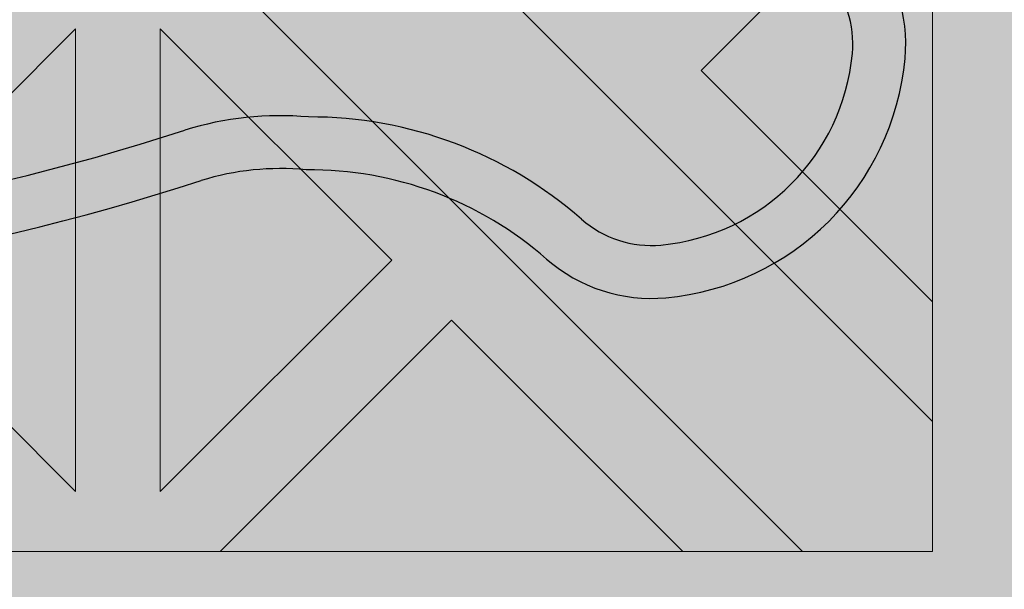
# Model space of a CAD drawing. Units: inches. Extents: x 844 to 2234, y 346 to 1084.
# Tile 10 of 93: x 1124.57 to 1127.536, y 686.542 to 688.258. Entities that reach past the tile are written whole.
import ezdxf

# ---------------------------------------------------------------- set-up
doc = ezdxf.new("R2010")
doc.units = ezdxf.units.IN
doc.header["$MEASUREMENT"] = 0
for name, color, linetype, lineweight in [('A-ANNO-DIMS', 2, 'Continuous', 18), ('furniture', 8, 'Continuous', 18), ('RA-AP-01$0$INT', 35, 'Continuous', 5)]:
    doc.layers.add(name, color=color, linetype=linetype, lineweight=lineweight)
doc.layers.add('RA-AP-01$0$FURN', color=3, linetype='Continuous')
doc.layers.add('RA-AP-01$0$WOOD', color=64, linetype='Continuous')
doc.styles.get("Standard").update_dxf_attribs({"font": 'arial.ttf'})
doc.dimstyles.get("Standard").update_dxf_attribs({"dimtxt": 6, "dimasz": 3, "dimexe": 0.18, "dimexo": 0.0625, "dimgap": 0.09, "dimtad": 0, "dimtih": 1, "dimtoh": 1, "dimdec": 1, "dimzin": 0, "dimdsep": 46, "dimlunit": 3, "dimtxsty": 'Standard', "dimblk": 'ARCHTICK', "dimcen": 0.09, "dimadec": 0, "dimazin": 0, "dimtfac": 1, "dimtdec": 1, "dimtofl": 0, "dimtmove": 0, "dimatfit": 3, "dimfxl": 1, "dimtolj": 1, "dimtzin": 0, "dimarcsym": 0})

# ---------------------------------------------------------------- blocks, each defined once
blk = doc.blocks.new('A$C18D01794')
at = {"layer": 'RA-AP-01$0$INT'}
blk.add_hatch(color=256, dxfattribs=at).paths.add_polyline_path([(4.505206456958071, -6.306712009588038), (5.305206456958072, -6.306712009588038), (5.305206456958072, -7.106712009588038), (5.255206456951893, -7.10671200958804), (5.25520645694868, -6.356712009605972), (4.555206456959269, -6.356712009587461), (4.555206456956052, -7.106712009588038), (4.505206456958073, -7.106712009588038)])
h = blk.add_hatch(color=256, dxfattribs=at)
h.paths.add_polyline_path([(4.585917135068449, -6.356712009588271), (4.555206456959269, -6.35671200958746), (4.555206456959137, -6.387422687716308), (4.874495778835233, -6.706712009592356), (4.90520645695423, -6.676001331474049)])
h.paths.add_polyline_path([(5.255206456948813, -6.387422687716306), (5.255206456948682, -6.356712009605972), (5.224495778822613, -6.356712009605161), (4.905206456953498, -6.676001331474273), (4.935917135072151, -6.706712009592924)])
h.paths.add_polyline_path([(4.935917135072559, -6.706712009592068), (4.905206456953564, -6.737422687710376), (5.255206456951813, -7.087422687708613), (5.255206456951549, -7.026001331471008)])
h.paths.add_polyline_path([(4.555206456956399, -7.026001331471013), (4.555206456956134, -7.087422687708616), (4.905206456953821, -6.737422687710943), (4.874495778835166, -6.70671200959229)])
h = blk.add_hatch(color=256, dxfattribs=at)
h.paths.add_polyline_path([(4.585917135068448, -6.356712009588273), (4.614201406330596, -6.356712009589021), (4.668846067270487, -6.411356670531338), (4.723490728212344, -6.356712009591912), (4.771774999457151, -6.35671200959319), (4.826419660396886, -6.411356670535356), (4.862780050090322, -6.374996280843536), (4.844495778842715, -6.356712009595112), (4.862780050090411, -6.356712009595595), (4.905206456960182, -6.399138416468211), (4.947632863832445, -6.356712009597838), (4.965917135079675, -6.356712009598322), (4.947632863831759, -6.374996280845421), (4.983993253523576, -6.411356670538857), (5.038637914464627, -6.356712009600247), (5.08692218571208, -6.356712009601523), (5.141566846649976, -6.411356670541852), (5.196211507589851, -6.356712009604411), (5.224495778822615, -6.356712009605161), (4.905206456953975, -6.676001331473793)])
h.paths.add_polyline_path([(4.895206456956031, -6.637717060225675), (4.895206456958921, -6.528427738347902), (4.840561796018589, -6.583072399285802)], flags=16)
h.paths.add_polyline_path([(4.915206456955638, -6.637717060226121), (4.969851117895509, -6.583072399288678), (4.915206456957609, -6.528427738348344)], flags=16)
h.paths.add_polyline_path([(4.826419660395175, -6.568930263661755), (4.881064321335613, -6.514285602723745), (4.771774999456703, -6.514285602720857)], flags=16)
h.paths.add_polyline_path([(4.983993253519558, -6.568930263665262), (5.038637914460456, -6.514285602726792), (4.929348592581548, -6.514285602724816)], flags=16)
h.paths.add_polyline_path([(4.881064321336025, -6.494285602723742), (4.826419660397532, -6.439640941782821), (4.771774999457062, -6.494285602720859)], flags=16)
h.paths.add_polyline_path([(4.929348592582019, -6.494285602724817), (5.038637914460982, -6.494285602726792), (4.983993253522945, -6.439640941786327)], flags=16)
h.paths.add_polyline_path([(4.895206456960191, -6.480143467100443), (4.895206456962115, -6.407422687715913), (4.876922185715016, -6.389138416467584), (4.840561796021581, -6.425498806159401)], flags=16)
h.paths.add_polyline_path([(4.915206456958487, -6.480143467100889), (4.969851117899527, -6.425498806162279), (4.933490728206909, -6.389138416468043), (4.9152064569598, -6.40742268771434)], flags=16)
h.paths.add_polyline_path([(4.757632863832376, -6.480143467096812), (4.812277524772842, -6.425498806158772), (4.757632863834348, -6.370854145217844)], flags=16)
h.paths.add_polyline_path([(4.737632863832376, -6.480143467096286), (4.737632863834348, -6.370854145217375), (4.682988202893906, -6.425498806155385)], flags=16)
h.paths.add_polyline_path([(5.05278005008503, -6.480143467103376), (5.052780050087917, -6.370854145224413), (4.998135389146995, -6.425498806162908)], flags=16)
h.paths.add_polyline_path([(5.072780050085024, -6.480143467103744), (5.127424711025931, -6.42549880616527), (5.072780050087916, -6.370854145224832)], flags=16)
h.paths.add_polyline_path([(4.935917135072783, -6.706712009592292), (5.255206456948811, -6.387422687716309), (5.255206456948932, -6.415706958964177), (5.200561796010279, -6.470351619902839), (5.255206456949403, -6.524996280841948), (5.25520645694961, -6.5732805520894), (5.200561796009787, -6.627925213029239), (5.236922185702417, -6.664285602721864), (5.255206456949919, -6.646001331474357), (5.255206456949998, -6.664285602721898), (5.212780050078687, -6.706712009592262), (5.25520645695036, -6.749138416463932), (5.255206456950438, -6.767422687711313), (5.236922185702424, -6.749138416463297), (5.200561796009796, -6.785498806155928), (5.255206456950753, -6.840143467096874), (5.25520645695096, -6.888427738341682), (5.200561796010322, -6.943072399282328), (5.255206456951428, -6.997717060223427), (5.255206456951547, -7.026001331471006)])
h.paths.add_polyline_path([(5.042988202883395, -6.785498806155427), (5.097632863823085, -6.840143467095101), (5.097632863822622, -6.730854145216193)], flags=16)
h.paths.add_polyline_path([(5.028846067259663, -6.771356670531693), (5.083490728198774, -6.716712009592573), (4.974201406321001, -6.716712009593042)], flags=16)
h.paths.add_polyline_path([(5.117632863823087, -6.840143467095186), (5.172277524762331, -6.785498806155926), (5.11763286382262, -6.730854145216225)], flags=16)
h.paths.add_polyline_path([(5.08349072819877, -6.696712009593886), (5.028846067259652, -6.642067348654775), (4.974201406320998, -6.696712009593438)], flags=16)
h.paths.add_polyline_path([(5.131774999446817, -6.854285602718917), (5.186419660386065, -6.799640941779662), (5.241064321325782, -6.854285602719365)], flags=17)
h.paths.add_polyline_path([(5.131774999446228, -6.716712009592374), (5.186419660386065, -6.771356670532194), (5.222780050079488, -6.734996280838764), (5.204495778832781, -6.716712009592063)], flags=16)
h.paths.add_polyline_path([(5.097632863822613, -6.682569873970264), (5.097632863823061, -6.573280552091354), (5.042988202883383, -6.627925213031044)], flags=16)
h.paths.add_polyline_path([(5.131774999446899, -6.874285602718915), (5.241064321325809, -6.874285602719364), (5.186419660386591, -6.928930263658598)], flags=17)
h.paths.add_polyline_path([(5.131774999446226, -6.696712009594078), (5.204495778830767, -6.696712009594374), (5.22278005007868, -6.67842773834687), (5.186419660386049, -6.642067348654249)], flags=16)
h.paths.add_polyline_path([(5.11763286382262, -6.682569873970225), (5.17227752476232, -6.627925213030515), (5.117632863823064, -6.573280552091267)], flags=16)
h.paths.add_polyline_path([(5.186419660386069, -6.613783077405491), (5.241064321325754, -6.559138416465795), (5.131774999446791, -6.559138416466263)], flags=16)
h.paths.add_polyline_path([(5.131774999446872, -6.539138416466263), (5.24106432132578, -6.539138416465794), (5.186419660386554, -6.484493755526573)], flags=16)
h.paths.add_polyline_path([(5.255206456951811, -7.08742268770861), (5.255206456951895, -7.106712009588038), (4.555206456956052, -7.106712009588038), (4.555206456956136, -7.087422687708617), (4.905206456953973, -6.737422687710788)])
h.paths.add_polyline_path([(4.983993253513404, -6.8444937555241), (4.92934859257295, -6.899138416462108), (5.03863791445186, -6.899138416465014)], flags=16)
h.paths.add_polyline_path([(4.969851117889988, -6.83035161990006), (4.915206456952556, -6.775706958960171), (4.915206456949648, -6.884996280837944)], flags=16)
h.paths.add_polyline_path([(4.929348592572535, -6.919138416462105), (4.983993253511019, -6.973783077403037), (5.038637914451496, -6.919138416465012)], flags=16)
h.paths.add_polyline_path([(5.052780050074912, -6.93328055208906), (4.998135389134438, -6.987925213027088), (5.052780050072919, -7.042569873968025)], flags=16)
h.paths.add_polyline_path([(5.07278005007491, -6.933280552089588), (5.072780050072918, -7.042569873968497), (5.127424711013374, -6.987925213030498)], flags=16)
h.paths.add_polyline_path([(4.89520645695295, -6.775706958959721), (4.840561796013067, -6.830351619897157), (4.895206456950961, -6.884996280837494)], flags=16)
h.paths.add_polyline_path([(4.915206456948365, -6.933280552085403), (4.915206456946434, -7.006001331471951), (4.933490728192729, -7.024285602719066), (4.969851117886972, -6.987925213026453)], flags=16)
h.paths.add_polyline_path([(4.881064321327021, -6.899138416461022), (4.82641966038902, -6.84449375552057), (4.771774999448108, -6.899138416459029)], flags=16)
h.paths.add_polyline_path([(4.895206456950073, -6.933280552084951), (4.840561796009022, -6.987925213023558), (4.876922185700835, -7.024285602716997), (4.895206456948749, -7.006001331469487)], flags=16)
h.paths.add_polyline_path([(4.983993253510392, -7.0020673486505), (4.947632863816944, -7.038427738342319), (4.965917135064043, -7.05671200959023), (5.038637914448995, -7.056712009591555)], flags=16)
h.paths.add_polyline_path([(4.881064321326543, -6.91913841646102), (4.771774999447578, -6.919138416459031), (4.826419660385607, -6.973783077399508)], flags=16)
h.paths.add_polyline_path([(4.905206456946447, -7.014285602717636), (4.862780050074785, -7.056712009588352), (4.947632863816685, -7.056712009589775)], flags=16)
h.paths.add_polyline_path([(5.14156684663679, -7.002067348654549), (5.086922185696452, -7.056712009592438), (5.196211507574223, -7.056712009594425)], flags=16)
h.paths.add_polyline_path([(4.8264196603837, -7.002067348646972), (4.771774999442643, -7.056712009585575), (4.8444957788276, -7.056712009587508), (4.862780050075511, -7.038427738340416)], flags=16)
h.paths.add_polyline_path([(4.812277524760289, -6.98792521302292), (4.757632863822258, -6.933280552082447), (4.757632863819352, -7.042569873961408)], flags=16)
h.paths.add_polyline_path([(4.73763286382226, -6.933280552082079), (4.682988202881349, -6.987925213020536), (4.737632863819352, -7.04256987396099)], flags=16)
h.paths.add_polyline_path([(4.723490728195188, -7.056712009584289), (4.668846067257299, -7.002067348643949), (4.614201406317417, -7.056712009581383)], flags=16)
h.paths.add_polyline_path([(4.597632863829262, -6.706712009592262), (4.555206456957951, -6.664285602721896), (4.555206456958029, -6.646001331474357), (4.573490728205535, -6.664285602721864), (4.609851117898167, -6.627925213029238), (4.555206456958338, -6.573280552089402), (4.555206456958546, -6.524996280841952), (4.60985111789767, -6.470351619902839), (4.555206456959015, -6.415706958964177), (4.555206456959138, -6.387422687716309), (4.874495778835167, -6.70671200959229), (4.5552064569564, -7.026001331471015), (4.555206456956523, -6.997717060223433), (4.609851117897629, -6.94307239928233), (4.555206456956988, -6.888427738341681), (4.555206456957198, -6.840143467096881), (4.609851117898153, -6.78549880615593), (4.573490728205528, -6.749138416463297), (4.555206456957507, -6.76742268771132), (4.555206456957585, -6.749138416463933)])
h.paths.add_polyline_path([(4.712780050085332, -6.730854145216195), (4.712780050084863, -6.840143467095105), (4.767424711024555, -6.785498806155427)], flags=16)
h.paths.add_polyline_path([(4.726922185709173, -6.716712009592573), (4.781566846648288, -6.771356670531693), (4.836211507586949, -6.716712009593043)], flags=16)
h.paths.add_polyline_path([(4.692780050085327, -6.730854145216225), (4.638135389145619, -6.785498806155928), (4.692780050084865, -6.840143467095185)], flags=16)
h.paths.add_polyline_path([(4.726922185709182, -6.696712009593886), (4.836211507586949, -6.696712009593436), (4.7815668466483, -6.642067348654773)], flags=16)
h.paths.add_polyline_path([(4.678637914461726, -6.71671200959237), (4.605917135075169, -6.716712009592063), (4.587632863828464, -6.734996280838766), (4.623993253521887, -6.771356670532195)], flags=16)
h.paths.add_polyline_path([(4.712780050085336, -6.68256987397026), (4.767424711024568, -6.627925213031042), (4.71278005008489, -6.573280552091352)], flags=16)
h.paths.add_polyline_path([(4.678637914461726, -6.696712009594076), (4.623993253521899, -6.642067348654247), (4.587632863829271, -6.67842773834687), (4.605917135077185, -6.696712009594376)], flags=16)
h.paths.add_polyline_path([(4.692780050085336, -6.682569873970228), (4.692780050084889, -6.573280552091267), (4.638135389145632, -6.627925213030515)], flags=16)
h.paths.add_polyline_path([(4.623993253521885, -6.799640941779662), (4.678637914461131, -6.854285602718915), (4.56934859258217, -6.854285602719365)], flags=17)
h.paths.add_polyline_path([(4.623993253521901, -6.613783077405509), (4.678637914461158, -6.559138416466263), (4.569348592582195, -6.559138416465795)], flags=16)
h.paths.add_polyline_path([(4.678637914461051, -6.874285602718915), (4.623993253521361, -6.928930263658598), (4.569348592582143, -6.874285602719364)], flags=17)
h.paths.add_polyline_path([(4.678637914461076, -6.539138416466263), (4.623993253521399, -6.484493755526573), (4.569348592582167, -6.539138416465796)], flags=16)
h = blk.add_hatch(color=256, dxfattribs=at)
h.paths.add_polyline_path([(4.969851117891331, -6.583072399286455), (4.915206456952669, -6.63771706022511), (4.915206456952222, -6.528427738347337)])
h.paths.add_polyline_path([(4.895206456953064, -6.637717060225108), (4.840561796014413, -6.583072399286448), (4.895206456953533, -6.528427738347335)])
h.paths.add_polyline_path([(4.826419660390684, -6.568930263662714), (4.771774999451003, -6.514285602723024), (4.881064321329913, -6.514285602723489)])
h.paths.add_polyline_path([(4.881064321329884, -6.494285602723492), (4.771774999450921, -6.494285602723024), (4.82641966039018, -6.439640941783778)])
h.paths.add_polyline_path([(4.895206456953734, -6.48014346709988), (4.840561796013912, -6.425498806160046), (4.876922185707337, -6.389138416466622), (4.895206456954043, -6.40742268771333)])
h.paths.add_polyline_path([(4.862780050082808, -6.374996280843689), (4.826419660390178, -6.411356670536314), (4.771774999450351, -6.356712009596481), (4.844495778835303, -6.356712009596181)])
h.paths.add_polyline_path([(4.812277524766446, -6.425498806160041), (4.757632863827191, -6.480143467099289), (4.757632863826741, -6.370854145220329)])
h.paths.add_polyline_path([(4.737632863827191, -6.480143467099214), (4.682988202887508, -6.425498806159518), (4.737632863826743, -6.370854145220299)])
h.paths.add_polyline_path([(4.668846067263777, -6.41135667053579), (4.614201406325123, -6.356712009597128), (4.723490728202894, -6.356712009596675)])
h.paths.add_polyline_path([(4.905206456953846, -6.399138416467422), (4.862780050082654, -6.356712009596229), (4.947632863824561, -6.356712009595756)])
h.paths.add_polyline_path([(4.915206456952028, -6.480143467099882), (4.91520645695173, -6.407422687715346), (4.933490728199234, -6.389138416467428), (4.96985111789186, -6.425498806160055)])
h.paths.add_polyline_path([(5.038637914454841, -6.494285602723048), (4.929348592575874, -6.494285602723497), (4.983993253515593, -6.439640941783787)])
h.paths.add_polyline_path([(4.983993253515065, -6.568930263662725), (4.929348592575849, -6.514285602723495), (5.038637914454755, -6.514285602723045)])
h.paths.add_polyline_path([(5.052780050079843, -6.480143467099317), (4.998135389140595, -6.425498806160058), (5.052780050080309, -6.370854145220356)])
h.paths.add_polyline_path([(4.983993253516868, -6.411356670536324), (4.947632863824241, -6.374996280843694), (4.965917135071747, -6.356712009596188), (5.038637914456701, -6.356712009596504)])
h.paths.add_polyline_path([(5.127424711019533, -6.425498806159557), (5.072780050079843, -6.480143467099239), (5.07278005008031, -6.370854145220326)])
h.paths.add_polyline_path([(5.141566846643269, -6.411356670535829), (5.086922185704154, -6.356712009596707), (5.196211507581929, -6.356712009597176)])
h = blk.add_hatch(color=256, dxfattribs=at)
h.paths.add_polyline_path([(5.028846067259997, -6.642067348655121), (4.974201406321342, -6.696712009593783), (5.083490728199115, -6.69671200959423)])
h.paths.add_polyline_path([(4.974201406321344, -6.716712009593388), (5.028846067260004, -6.771356670532039), (5.083490728199117, -6.716712009592919)])
h.paths.add_polyline_path([(5.042988202883738, -6.785498806155768), (5.097632863823428, -6.840143467095449), (5.097632863822963, -6.73085414521654)])
h.paths.add_polyline_path([(5.117632863822961, -6.730854145216568), (5.117632863823428, -6.840143467095531), (5.172277524762674, -6.785498806156272)])
h.paths.add_polyline_path([(5.131774999446572, -6.716712009592718), (5.186419660386406, -6.77135667053254), (5.222780050079831, -6.734996280839116), (5.204495778833122, -6.716712009592409)])
h.paths.add_polyline_path([(5.236922185702764, -6.749138416463644), (5.200561796010139, -6.785498806156274), (5.255206456949971, -6.840143467096101), (5.255206456950271, -6.76742268771115)])
h.paths.add_polyline_path([(5.186419660386412, -6.799640941780006), (5.131774999447164, -6.854285602719262), (5.241064321326123, -6.854285602719711)])
h.paths.add_polyline_path([(5.131774999447238, -6.874285602719261), (5.186419660386934, -6.928930263658944), (5.241064321326153, -6.874285602719709)])
h.paths.add_polyline_path([(5.200561796010663, -6.943072399282675), (5.255206456949324, -6.997717060221329), (5.255206456949777, -6.888427738343558)])
h.paths.add_polyline_path([(5.21278005007903, -6.706712009592607), (5.255206456950223, -6.749138416463798), (5.255206456950696, -6.664285602721891)])
h.paths.add_polyline_path([(5.13177499944657, -6.696712009594424), (5.204495778831106, -6.696712009594723), (5.222780050079024, -6.678427738347219), (5.186419660386397, -6.642067348654592)])
h.paths.add_polyline_path([(5.117632863823405, -6.573280552091611), (5.117632863822955, -6.682569873970578), (5.172277524762665, -6.627925213030859)])
h.paths.add_polyline_path([(5.042988202883727, -6.627925213031387), (5.097632863822957, -6.682569873970603), (5.097632863823407, -6.573280552091697)])
h.paths.add_polyline_path([(5.131774999447135, -6.559138416466609), (5.186419660386394, -6.613783077405857), (5.241064321326097, -6.559138416466144)])
h.paths.add_polyline_path([(5.200561796010128, -6.627925213029584), (5.236922185702758, -6.664285602722211), (5.255206456950264, -6.646001331474705), (5.255206456949948, -6.573280552089752)])
h.paths.add_polyline_path([(5.186419660386895, -6.484493755526919), (5.131774999447213, -6.539138416466609), (5.241064321326127, -6.539138416466142)])
h.paths.add_polyline_path([(5.200561796010624, -6.470351619903183), (5.255206456949745, -6.524996280842298), (5.255206456949276, -6.415706958964523)])
for p, q in [((4.555206456959269, -6.356712009587461), (5.255206456948681, -6.356712009605972)), ((4.905206456953975, -6.676001331473793), (5.224495778822613, -6.356712009605161)), ((5.086922185712082, -6.356712009601526), (5.141566846649976, -6.411356670541854)), ((5.196211507589851, -6.356712009604413), (5.141566846649976, -6.411356670541854)), ((5.255206456951895, -7.106712009588038), (5.255206456948681, -6.356712009605972)), ((5.052780050087917, -6.370854145224413), (4.998135389146995, -6.425498806162908)), ((5.052780050085028, -6.480143467103376), (5.052780050087917, -6.370854145224413)), ((5.072780050085028, -6.48014346710374), (5.072780050087916, -6.37085414522483)), ((5.072780050087916, -6.37085414522483), (5.127424711025931, -6.42549880616527)), ((4.935917135072783, -6.706712009592292), (5.255206456948813, -6.387422687716307)), ((5.255206456948934, -6.415706958964177), (5.200561796010281, -6.470351619902839)), ((5.052780050085028, -6.480143467103376), (4.998135389146995, -6.425498806162908)), ((5.12742471102593, -6.425498806165272), (5.072780050085028, -6.48014346710374)), ((5.255206456949399, -6.524996280841946), (5.200561796010281, -6.470351619902839))]:
    blk.add_line(p, q, dxfattribs=at)
blk = doc.blocks.new('A$C32926AE1')
at = {"layer": 'RA-AP-01$0$WOOD'}
h = blk.add_hatch(color=256, dxfattribs=at)
h.dxf.hatch_style = 1
h.paths.add_polyline_path([(5.157430609644524, 4.573483066760929, -0.1009492694046607), (5.155401577623758, 4.593365984175333, -0.1842662638101597), (5.172249623284174, 4.638795604568598, 0.2056608120311276), (5.179560981299304, 4.661316324430096, 0.3614336704623542), (5.134352340494423, 4.706524965234944, 0.2056608120311297), (5.111831620632933, 4.699213607219793, -0.1842662638101113), (5.066402000239693, 4.682365561559342, -0.1055311479399994), (5.045656153913092, 4.68467289944697, 0.1567636581983829), (4.763886414745334, 4.684672899446966, -0.1055311479399895), (4.743140568418733, 4.68236556155934, -0.1842662638100833), (4.6977109480255, 4.69921360721979, 0.2056608120302612), (4.675190228164109, 4.706524965234949, 0.3614336704708441), (4.629981587358889, 4.66131632442871, 0.2056608120245944), (4.637292945374126, 4.638795604567974, -0.1842662638101024), (4.654140991034615, 4.59336598417475, -0.1009492694055169), (4.652111959013835, 4.573483066760181, 0.021410119221476), (4.629748025606143, 4.156712009541676, 0.0214101192214795), (4.652111959013809, 3.739940952323101, -0.1009492694059586), (4.654140991034615, 3.720058034908448, -0.1842662638100975), (4.637292945374126, 3.674628414515226, 0.2056608120245705), (4.629981587358889, 3.652107694654492, 0.3614336704708879), (4.675190228164113, 3.606899053848249, 0.2056608120302384), (4.697710948025501, 3.614210411863408, -0.1842662638100995), (4.743140568418738, 3.63105845752386, -0.1055311479402541), (4.763886414745388, 3.628751119636215, 0.1567636581983776), (5.045656153913137, 3.628751119636244, -0.1055311479397538), (5.066402000239692, 3.631058457523857, -0.1842662638101067), (5.111831620632931, 3.614210411863407, 0.2056608120310924), (5.134352340494417, 3.606899053848256, 0.3614336704624001), (5.179560981299307, 3.652107694653103, 0.2056608120311314), (5.172249623284175, 3.6746284145146, -0.1842662638101402), (5.155401577623758, 3.72005803490786, -0.1009492694051366), (5.15743060964455, 3.739940952322354, 0.0214101192215073), (5.179794543052287, 4.156712009541468, 0.0214101192215252)])
h.paths.add_polyline_path([(4.639748609479751, 4.156712009541513, 0.0213537860821624), (4.661970494867118, 3.741887061152232, -0.094075836301374), (4.664143710413708, 3.7196126951003, -0.1824818158568985), (4.644813765429836, 3.668037719127816, 0.2056608120245319), (4.639939526753007, 3.653023905887301, 0.3614336704710246), (4.676106439397173, 3.616856993242342, 0.2056608120302234), (4.691120252638095, 3.621731231919122, -0.1824818158602558), (4.742695228611606, 3.641061176902986, -0.1029891339458722), (4.766991894714349, 3.638256818950944, 0.156709409989566), (5.042550673941472, 3.638256818950105, -0.102989133958497), (5.066847340047078, 3.641061176902949, -0.1824818158594995), (5.118422316020358, 3.621731231919103, 0.2056608120311416), (5.133436129261316, 3.616856993242346, 0.3614336704621468), (5.169603041905217, 3.653023905886178, 0.2056608120310986), (5.164728803228477, 3.668037719127177, -0.1824818158565612), (5.145398858244737, 3.719612695099578, -0.0940758363009313), (5.147572073791232, 3.741887061151398, 0.0213537860822023), (5.169793959178681, 4.156712009541451, 0.0213537860822226), (5.147572073791203, 4.571536957931898, -0.0940758363005034), (5.145398858244737, 4.59381132398362, -0.1824818158565587), (5.164728803228476, 4.645386299956021, 0.2056608120311045), (5.169603041905216, 4.66040011319702, 0.3614336704621845), (5.133436129261313, 4.696567025840856, 0.2056608120310773), (5.118422316020359, 4.691692787164098, -0.182481815859508), (5.066847340047078, 4.67236284218025, -0.1029891339584606), (5.04255067394148, 4.675167200133092, 0.156709409989566), (4.766991894714357, 4.675167200132257, -0.1029891339458842), (4.742695228611611, 4.672362842180213, -0.1824818158602725), (4.691120252638095, 4.691692787164077, 0.2056608120302152), (4.676106439397174, 4.696567025840858, 0.3614336704710363), (4.639939526753005, 4.660400113195899, 0.2056608120245495), (4.644813765429837, 4.645386299955384, -0.1824818158568934), (4.664143710413708, 4.593811323982902, -0.0940758363009187), (4.661970494867149, 4.571536957931074, 0.021353786082177)], flags=16)
h.paths.add_polyline_path([(5.129794543052235, 4.432167055276933, -0.0141661062790638), (5.130152669293814, 4.156927903047693, -0.0141661062790647), (5.129794543052234, 3.881688750818433, -0.0785247771143638), (5.10979738006795, 3.755143611847103, 0.0945969212073497), (5.105408519571111, 3.717898134952927, 0.1043170707844957), (5.116074640131521, 3.670385395016088, 0.1043170707864965), (5.068561900193738, 3.681051515576561, 0.09459692119553), (5.031316423304057, 3.676662655080835, -0.1580239521427272), (4.778226145355827, 3.676662655080367, 0.0945969211986668), (4.740980668464973, 3.681051515576592, 0.1043170707882822), (4.693467928526415, 3.670385395015844, 0.1043170707867916), (4.704134049087309, 3.717898134953662, 0.0945969211972894), (4.69974518859162, 3.755143611844042, -0.0785247771163196), (4.679748025606343, 3.881688750818406, -0.0141661062790663), (4.679389899364763, 4.156927903047693, -0.0141661062790672), (4.679748025606343, 4.432167055276998, -0.0785247771163064), (4.699745188591625, 4.55871219425134, 0.094596921197333), (4.704134049087308, 4.595957671141738, 0.1043170707867205), (4.693467928526416, 4.643470411079523, 0.1043170707882628), (4.740980668464965, 4.632804290518776, 0.0945969211988114), (4.778226145355874, 4.637193151015016, -0.158023952142669), (5.031316423304015, 4.637193151014546, 0.0945969211956361), (5.068561900193736, 4.632804290518806, 0.1043170707864979), (5.11607464013152, 4.643470411079278, 0.1043170707844617), (5.105408519571112, 4.595957671142455, 0.0945969212074597), (5.109797380067959, 4.558712194248236, -0.0785247771143467)], flags=0)
h.paths.add_polyline_path([(5.119794532311105, 4.432259799204851, -0.0142000800617244), (5.120156169157484, 4.156927903047701, -0.0142000800617277), (5.119794532311105, 3.881596006890482, -0.0784894509520253), (5.100273383573699, 3.758192358677797, 0.0940138827242913), (5.095413455884425, 3.717477693979438, 0.0606271852308753), (5.099615656341024, 3.686844378806616, 0.0606271852322524), (5.068982341167493, 3.691046579263239, 0.0940138827010453), (5.028267676478798, 3.686186651576848, -0.1580706864508061), (4.781274892180912, 3.686186651576435, 0.0940138827026903), (4.740560227491556, 3.691046579263279, 0.0606271852339895), (4.709926912317155, 3.686844378806508, 0.0606271852329405), (4.714129112773991, 3.717477693980356, 0.094013882701304), (4.709269185087677, 3.758192358669163, -0.0784894509577193), (4.689748036347473, 3.881596006890469, -0.014200080061729), (4.689386399501094, 4.156927903047709, -0.0142000800617217), (4.689748036347473, 4.432259799204808, -0.078489450957724), (4.709269185087651, 4.555663447426125, 0.0940138827014585), (4.714129112773992, 4.596378112114996, 0.0606271852329731), (4.709926912317154, 4.62701142728886, 0.0606271852340196), (4.74056022749157, 4.622809226832087, 0.0940138827024997), (4.781274892180847, 4.627669154518912, -0.1580706864508359), (5.028267676478777, 4.627669154518526, 0.0940138827010946), (5.068982341167492, 4.622809226832129, 0.060627185232254), (5.099615656341024, 4.627011427288751, 0.0606271852308727), (5.095413455884425, 4.59637811211593, 0.0940138827241088), (5.100273383573675, 4.555663447417647, -0.0784894509520978)], flags=0)
h.paths.add_polyline_path([(5.06978912287499, 4.430218106756144, -0.014241683694547), (5.070173729147532, 4.156927903047672, -0.0142416836945458), (5.06978912287499, 3.883637699339223, -0.0800609523125196), (5.052662118612511, 3.773463122773442, 0.0526421978001116), (5.04590916754064, 3.740550867606997, 0.0526421977992423), (5.012996912374707, 3.73379791653534, -0.1583028414718258), (4.796545656286308, 3.73379791653451, 0.0526421978034211), (4.763633401117837, 3.740550867607021, 0.0526421978018622), (4.756880450045755, 3.773463122774558, -0.0800609523117106), (4.739753445783639, 3.883637699339268, -0.0142416836945435), (4.739368839511098, 4.156927903047671, -0.0142416836945477), (4.739753445783639, 4.430218106756155, -0.0800609523116345), (4.75688045004574, 4.540392683320762, 0.052642197801941), (4.763633401117837, 4.573304938488346, 0.0526421978035071), (4.796545656286361, 4.580057889560873, -0.1583028414717561), (5.012996912374669, 4.580057889560039, 0.0526421977993048), (5.04590916754064, 4.57330493848837, 0.0526421978002057), (5.052662118612529, 4.540392683321868, -0.080060952312477)], flags=0)
h.paths.add_polyline_path([(5.049789715110557, 4.43038092723357, -0.0143097550741839), (5.05018085590259, 4.156927903047715, -0.0143097550741854), (5.049789715110558, 3.883474878861827, -0.0800685599149176), (5.03362098255317, 3.779581877367999, 0.0306258898956367), (5.028241146483733, 3.758218888663947, 0.0306258898977031), (5.006878157778253, 3.75283905259408, -0.1583983521624096), (4.802664410878162, 3.752839052594731, 0.0306258898946014), (4.781301422174808, 3.758218888663924, 0.0306258898967912), (4.775921586105202, 3.779581877368794, -0.080068559914251), (4.759752853548071, 3.883474878861786, -0.0143097550741854), (4.759361712756037, 4.156927903047671, -0.0143097550741854), (4.759752853548071, 4.430380927233557, -0.0800685599142479), (4.775921586105193, 4.534273928726546, 0.0306258898968306), (4.781301422174808, 4.555636917431444, 0.0306258898945754), (4.802664410878143, 4.561016753500631, -0.1583983521624168), (5.006878157778244, 4.561016753501291, 0.0306258898977177), (5.028241146483733, 4.555636917431421, 0.0306258898958182), (5.03362098255321, 4.534273928727244, -0.080068559914796)], flags=0)
h.paths.add_polyline_path([(4.999766070382627, 4.428171244713864, -0.0143443147609634), (5.000198441819402, 4.156927903047689, -0.0143443147609612), (4.999766070382627, 3.885684561381556, -0.0784641635803329), (4.987356730658798, 3.799103304488872, -0.1506053783831347), (4.822185837999821, 3.79910330448882, -0.0784641635803318), (4.809776498276007, 3.885684561381509, -0.014344314760963), (4.809344126839227, 4.156927903047677, -0.0143443147609645), (4.809776498276007, 4.428171244713873, -0.0784641635803192), (4.822185837999822, 4.514752501606549, -0.1506053783831338), (4.987356730658798, 4.514752501606494, -0.078464163580285)], flags=0)
h.paths.add_polyline_path([(4.979755254238824, 4.42764379880488, -0.0143772539198268), (4.980205517789977, 4.156927903047693, -0.0143772539198275), (4.979755254238824, 3.886212007290489, -0.0689242507424422), (4.971183264704897, 3.815276770442801, -0.1296645318904179), (4.838359303953726, 3.815276770442746, -0.0689242507424186), (4.829787314419809, 3.886212007290419, -0.0143772539198292), (4.829337050868653, 4.156927903047653, -0.0143772539198325), (4.829787314419809, 4.427643798804946, -0.0689242507424211), (4.838359303953725, 4.498579035652621, -0.1296645318904187), (4.971183264704897, 4.498579035652565, -0.0689242507424401)], flags=0)
h = blk.add_hatch(color=256, dxfattribs=at)
h.dxf.hatch_style = 1
h.paths.add_polyline_path([(5.145398858244737, 4.59381132398362, -0.1824818158565616), (5.164728803228476, 4.645386299956021, 0.2056608120311045), (5.169603041905216, 4.66040011319702, 0.3614336704621845), (5.133436129261313, 4.696567025840856, 0.2056608120310773), (5.118422316020359, 4.691692787164098, -0.182481815859508), (5.066847340047078, 4.67236284218025, -0.1029891339584606), (5.04255067394148, 4.675167200133092, 0.156709409989566), (4.766991894714357, 4.675167200132257, -0.1029891339458842), (4.742695228611611, 4.672362842180213, -0.1824818158602725), (4.691120252638095, 4.691692787164077, 0.2056608120302152), (4.676106439397174, 4.696567025840858, 0.3614336704710363), (4.639939526753005, 4.660400113195899, 0.2056608120245495), (4.644813765429837, 4.645386299955384, -0.1824818158568934), (4.664143710413708, 4.593811323982902, -0.0940758363009187), (4.661970494867149, 4.571536957931074, 0.0213537860821772), (4.639748609479751, 4.156712009541507, 0.0213537860821625), (4.661970494867119, 3.741887061152226, -0.0940758363013071), (4.664143710413708, 3.719612695100309, -0.1824818158569294), (4.644813765429836, 3.668037719127816, 0.2056608120245319), (4.639939526753007, 3.653023905887301, 0.3614336704710246), (4.676106439397173, 3.616856993242342, 0.2056608120302234), (4.691120252638095, 3.621731231919122, -0.1824818158602558), (4.742695228611606, 3.641061176902986, -0.1029891339458722), (4.766991894714349, 3.638256818950944, 0.156709409989566), (5.042550673941472, 3.638256818950105, -0.102989133958497), (5.066847340047078, 3.641061176902949, -0.1824818158594995), (5.118422316020358, 3.621731231919103, 0.2056608120311416), (5.133436129261316, 3.616856993242346, 0.3614336704621468), (5.169603041905217, 3.653023905886178, 0.2056608120310986), (5.164728803228477, 3.668037719127177, -0.1824818158565612), (5.145398858244737, 3.719612695099578, -0.0940758363009313), (5.147572073791232, 3.741887061151398, 0.0213537860822023), (5.169793959178681, 4.156712009541451, 0.0213537860822226), (5.147572073791203, 4.571536957931898, -0.0940758363004996)])
h.paths.add_polyline_path([(5.109797380067958, 4.55871219424824, -0.0785247771143472), (5.129794543052234, 4.432167055276936, -0.0141661062790644), (5.130152669293814, 4.156927903047685, -0.014166106279066), (5.129794543052234, 3.881688750818401, -0.0785247771143517), (5.109797380067946, 3.755143611847092, 0.0945969212073132), (5.105408519571111, 3.717898134952929, 0.1043170707844995), (5.116074640131521, 3.670385395016088, 0.1043170707864965), (5.068561900193738, 3.681051515576561, 0.09459692119553), (5.031316423304057, 3.676662655080835, -0.1580239521427272), (4.778226145355827, 3.676662655080367, 0.0945969211986668), (4.740980668464973, 3.681051515576592, 0.1043170707882822), (4.693467928526415, 3.670385395015844, 0.1043170707867916), (4.704134049087309, 3.717898134953662, 0.0945969211972894), (4.69974518859162, 3.755143611844042, -0.0785247771163196), (4.679748025606343, 3.881688750818406, -0.0141661062790663), (4.679389899364763, 4.156927903047693, -0.0141661062790672), (4.679748025606343, 4.432167055276998, -0.0785247771163064), (4.699745188591625, 4.55871219425134, 0.094596921197333), (4.704134049087308, 4.595957671141738, 0.1043170707867205), (4.693467928526416, 4.643470411079523, 0.1043170707882628), (4.740980668464965, 4.632804290518776, 0.0945969211988114), (4.778226145355874, 4.637193151015016, -0.158023952142669), (5.031316423304015, 4.637193151014546, 0.0945969211956361), (5.068561900193736, 4.632804290518806, 0.1043170707864979), (5.11607464013152, 4.643470411079278, 0.1043170707844617), (5.105408519571112, 4.595957671142455, 0.0945969212074504)], flags=16)
h.paths.add_polyline_path([(5.100273383573655, 4.55566344741771, -0.0784894509521388), (5.119794532311105, 4.432259799204852, -0.0142000800617252), (5.120156169157484, 4.156927903047686, -0.014200080061726), (5.119794532311105, 3.881596006890502, -0.0784894509520446), (5.100273383573696, 3.758192358677786, 0.0940138827242721), (5.095413455884425, 3.717477693979436, 0.0606271852308692), (5.099615656341024, 3.686844378806616, 0.0606271852322522), (5.068982341167493, 3.691046579263239, 0.0940138827010453), (5.028267676478798, 3.686186651576848, -0.1580706864508061), (4.781274892180912, 3.686186651576435, 0.0940138827026903), (4.740560227491556, 3.691046579263279, 0.0606271852339895), (4.709926912317155, 3.686844378806508, 0.0606271852329405), (4.714129112773991, 3.717477693980356, 0.094013882701304), (4.709269185087677, 3.758192358669163, -0.0784894509577193), (4.689748036347473, 3.881596006890469, -0.014200080061729), (4.689386399501094, 4.156927903047709, -0.0142000800617217), (4.689748036347473, 4.432259799204808, -0.078489450957724), (4.709269185087651, 4.555663447426125, 0.0940138827014585), (4.714129112773992, 4.596378112114996, 0.0606271852329731), (4.709926912317154, 4.62701142728886, 0.0606271852340196), (4.74056022749157, 4.622809226832087, 0.0940138827024997), (4.781274892180847, 4.627669154518912, -0.1580706864508359), (5.028267676478777, 4.627669154518526, 0.0940138827010946), (5.068982341167492, 4.622809226832129, 0.060627185232254), (5.099615656341024, 4.627011427288751, 0.0606271852308727), (5.095413455884425, 4.59637811211593, 0.094013882723957)], flags=0)
h.paths.add_polyline_path([(5.04590916754064, 4.57330493848837, 0.0526421978002057), (5.052662118612529, 4.540392683321868, -0.0800609523124783), (5.06978912287499, 4.430218106756142, -0.0142416836945469), (5.070173729147532, 4.156927903047672, -0.0142416836945458), (5.06978912287499, 3.883637699339223, -0.0800609523125196), (5.052662118612511, 3.773463122773442, 0.0526421978001116), (5.04590916754064, 3.740550867606997, 0.0526421977992423), (5.012996912374707, 3.73379791653534, -0.1583028414718258), (4.796545656286308, 3.73379791653451, 0.0526421978034211), (4.763633401117837, 3.740550867607021, 0.0526421978018622), (4.756880450045755, 3.773463122774558, -0.0800609523117106), (4.739753445783639, 3.883637699339268, -0.0142416836945435), (4.739368839511098, 4.156927903047671, -0.0142416836945477), (4.739753445783639, 4.430218106756155, -0.0800609523116345), (4.75688045004574, 4.540392683320762, 0.052642197801941), (4.763633401117837, 4.573304938488346, 0.0526421978035071), (4.796545656286361, 4.580057889560873, -0.1583028414717561), (5.012996912374669, 4.580057889560039, 0.0526421977993048)], flags=0)
h.paths.add_polyline_path([(5.028241146483733, 4.555636917431422, 0.0306258898956949), (5.033620982553182, 4.534273928727329, -0.0800685599148649), (5.049789715110557, 4.430380927233569, -0.0143097550741839), (5.05018085590259, 4.156927903047715, -0.0143097550741854), (5.049789715110558, 3.883474878861827, -0.0800685599149176), (5.03362098255317, 3.779581877367999, 0.0306258898956367), (5.028241146483733, 3.758218888663947, 0.0306258898977031), (5.006878157778253, 3.75283905259408, -0.1583983521624096), (4.802664410878162, 3.752839052594731, 0.0306258898946014), (4.781301422174808, 3.758218888663924, 0.0306258898967912), (4.775921586105202, 3.779581877368794, -0.080068559914251), (4.759752853548071, 3.883474878861786, -0.0143097550741854), (4.759361712756037, 4.156927903047671, -0.0143097550741854), (4.759752853548071, 4.430380927233557, -0.0800685599142479), (4.775921586105193, 4.534273928726546, 0.0306258898968306), (4.781301422174808, 4.555636917431444, 0.0306258898945754), (4.802664410878143, 4.561016753500631, -0.1583983521624168), (5.006878157778244, 4.561016753501291, 0.0306258898977174)], flags=0)
h.paths.add_polyline_path([(4.987356730658798, 4.514752501606494, -0.0784641635803018), (4.999766070382627, 4.428171244713845, -0.0143443147609637), (5.000198441819402, 4.156927903047665, -0.0143443147609622), (4.999766070382628, 3.885684561381514, -0.0784641635802952), (4.987356730658797, 3.799103304488872, -0.1506053783831338), (4.822185837999821, 3.799103304488819, -0.0784641635803342), (4.809776498276007, 3.885684561381512, -0.0143443147609628), (4.809344126839227, 4.156927903047676, -0.0143443147609646), (4.809776498276007, 4.428171244713873, -0.0784641635803192), (4.822185837999822, 4.514752501606549, -0.1506053783831338)], flags=0)
h.paths.add_polyline_path([(4.971183264704897, 4.498579035652566, -0.0689242507424384), (4.979755254238824, 4.427643798804883, -0.0143772539198276), (4.980205517789977, 4.15692790304768, -0.0143772539198258), (4.979755254238823, 3.88621200729051, -0.0689242507424628), (4.971183264704897, 3.815276770442801, -0.129664531890417), (4.838359303953726, 3.815276770442746, -0.0689242507424186), (4.829787314419809, 3.886212007290419, -0.0143772539198292), (4.829337050868653, 4.156927903047653, -0.0143772539198325), (4.829787314419809, 4.427643798804946, -0.0689242507424211), (4.838359303953725, 4.498579035652621, -0.1296645318904187)], flags=0)
h = blk.add_hatch(dxfattribs=at)
h.set_pattern_fill('ANSI31', color=256, scale=0.05, style=0)
h.set_pattern_definition([(45, (0, 0), (-0.0044194173824159, 0.0044194173824159), [])])
h.paths.add_polyline_path([(5.130152669293814, 4.156927903047704, 0.0141661062790657), (5.129794543052234, 4.432167055276982, 0.0777827904001433), (5.110168979996553, 4.557559993161921, -0.0976515123401879), (5.105408519571111, 4.595957671142454, -0.1043170707844687), (5.116074640131522, 4.64347041107928), (5.099615656341024, 4.627011427288751, 0.0606271852308727), (5.095413455884425, 4.59637811211593, 0.0940138827241088), (5.100273383573675, 4.555663447417647, -0.0784894509520972), (5.119794532311105, 4.432259799204852, -0.0142000800617252), (5.120156169157484, 4.156927903047686, -0.014200080061726), (5.119794532311105, 3.881596006890502, -0.0784894509520446), (5.100273383573696, 3.758192358677786, 0.0940138827242721), (5.095413455884425, 3.717477693979436, 0.0606271852308692), (5.099615656341024, 3.686844378806616), (5.116074640131519, 3.67038539501609, -0.1043170707844594), (5.105408519571112, 3.717898134952912, -0.0976515123401594), (5.11016897999655, 3.756295812933435, 0.0777827904001654), (5.129794543052234, 3.881688750818409, 0.0141661062790665)])
h.paths.add_polyline_path([(5.030164222210597, 3.676291055149937, -0.0976515123472002), (5.068561900193739, 3.681051515576561, -0.1043170707864927), (5.116074640131521, 3.670385395016088), (5.099615656341024, 3.686844378806616, 0.0606271852322522), (5.068982341167493, 3.691046579263239, 0.0940138827010453), (5.028267676478798, 3.686186651576848, -0.1580706864508061), (4.781274892180912, 3.686186651576435, 0.0940138827026903), (4.740560227491556, 3.691046579263279, 0.0606271852339913), (4.709926912317154, 3.686844378806508), (4.693467928526416, 3.670385395015845, -0.1043170707882796), (4.740980668464973, 3.681051515576592, -0.0976515123427246), (4.779378346446416, 3.676291055150394, 0.156512506893803)])
h.paths.add_polyline_path([(4.689748036347473, 3.881596006890472, -0.014200080061729), (4.689386399501094, 4.156927903047712, -0.0142000800617195), (4.689748036347473, 4.432259799204768, -0.078489450957742), (4.709269185087648, 4.555663447426114, 0.0940138827014821), (4.714129112773992, 4.596378112114995, 0.0606271852329748), (4.709926912317154, 4.62701142728886), (4.693467928526414, 4.643470411079524, -0.1043170707867939), (4.704134049087309, 4.595957671141706, -0.09765151234893), (4.699373588660725, 4.557559993157876, 0.0777827903975372), (4.679748025606343, 4.432167055276987, 0.0141661062790675), (4.679389899364763, 4.156927903047675, 0.0141661062790641), (4.679748025606343, 3.88168875081843, 0.0777827903975637), (4.699373588660724, 3.756295812937497, -0.0976515123490278), (4.704134049087308, 3.717898134953629, -0.1043170707867196), (4.693467928526416, 3.670385395015845), (4.709926912317155, 3.686844378806508, 0.0606271852329413), (4.714129112773991, 3.717477693980357, 0.0940138827013084), (4.709269185087676, 3.758192358669166, -0.0784894509577192)])
h.paths.add_polyline_path([(4.779378346446434, 4.63756475094498, -0.0976515123427943), (4.740980668464964, 4.632804290518776, -0.1043170707882609), (4.693467928526416, 4.643470411079523), (4.709926912317154, 4.62701142728886, 0.0606271852340196), (4.74056022749157, 4.622809226832087, 0.0940138827024997), (4.781274892180847, 4.627669154518912, -0.1580706864508359), (5.028267676478777, 4.627669154518526, 0.0940138827010946), (5.068982341167492, 4.622809226832129, 0.060627185232254), (5.099615656341024, 4.627011427288751), (5.116074640131521, 4.643470411079279, -0.1043170707865022), (5.068561900193735, 4.632804290518806, -0.0976515123475899), (5.030164222210446, 4.637564750945479, 0.1565125068936924)])
for centre, radius, start, end in [((4.904771284329219, 4.067062675376636), 0.4103971832811756, 252.0403002450644, 287.9596997551364), ((5.149687163117039, 3.654856328352376), 0.0300000000000001, 354.7431240045364, 41.22894907959901), ((5.14968716311704, 3.654856328352378), 0.0199999999999982, 354.7431240045299, 41.22894907959565), ((5.129771284329002, 3.656688750818565), 0.0399999999998586, 275.2568759945327, 354.7431240047909), ((5.129771284329024, 3.656688750818544), 0.0499999999998358, 275.2568759945053, 354.7431240047624), ((5.061434214607045, 3.58130585853738), 0.0600000000000002, 84.82380783952524, 107.4061270451724), ((5.067034653563934, 3.563091385939257), 0.0779700159630323, 48.77105092035808, 90.13764630098588), ((4.904771284329217, 4.067062675376635), 0.4503971832811742, 252.0623235132636, 287.9376764870612), ((5.06143421460707, 3.58130585853739), 0.0499999999999993, 84.29792923463329, 107.3556839752475), ((5.067034653563935, 3.563091385939262), 0.0679700159630267, 48.77105092035588, 90.5333070513694), ((4.904771284329219, 4.067062675376637), 0.4603971832811766, 252.0683908477148, 287.9316091522846), ((5.131603706795156, 3.636772872030479), 0.019999999999953, 228.7710509202994, 275.2568759942249), ((5.131603706795172, 3.636772872030527), 0.0299999999999995, 228.7710509203566, 275.2568759942798)]:
    blk.add_arc(centre, radius, start, end, dxfattribs=at)
blk = doc.blocks.new('A$C5D2F253E')
at = {"layer": 'RA-AP-01$0$FURN', "xscale": -0.7999999999883585, "yscale": 0.7999999999883585, "zscale": 0.8, "rotation": 90}
blk.add_blockref('A$C18D01794', (-5.687757199772477, 4.75791982714071), dxfattribs=at)
at = {"layer": 'RA-AP-01$0$WOOD', "rotation": 270}
blk.add_blockref('A$C32926AE1', (-4.161339601644158, 5.73852594588169), dxfattribs=at)
blk = doc.blocks.new('_ArchTick')
at = {"color": 0, "linetype": 'ByBlock', "const_width": 0.15}
blk.add_lwpolyline([(-0.5, -0.5), (0.5, 0.5)], dxfattribs=at)
blk = doc.blocks.new('*D144')
at = {"layer": 'A-ANNO-DIMS', "color": 0, "lineweight": -2, "transparency": 16777216}
for p, q in [((1096.615948, 439.3732739999999), (1096.615948, 1074.743301)), ((1143.115948, 492.373274), (1143.115948, 1074.743301)), ((1096.615948, 1074.563301), (1102.481950728513, 1074.563301)), ((1143.115948, 1074.563301), (1137.249945271487, 1074.563301))]:
    blk.add_line(p, q, dxfattribs=at)
at = {"layer": 'Defpoints', "color": 0, "transparency": 16777216}
for p in [(1143.115948, 1074.563301), (1143.115948, 492.3107739999999), (1096.615948, 439.3107739999999)]:
    blk.add_point(p, dxfattribs=at)
at = {"layer": 'A-ANNO-DIMS', "color": 0, "lineweight": -2, "transparency": 16777216, "xscale": 3, "yscale": 3, "zscale": 3, "rotation": 180}
blk.add_blockref('_ArchTick', (1096.615948, 1074.563301), dxfattribs=at)
at = {"layer": 'A-ANNO-DIMS', "color": 0, "lineweight": -2, "transparency": 16777216, "xscale": 3, "yscale": 3, "zscale": 3}
blk.add_blockref('_ArchTick', (1143.115948, 1074.563301), dxfattribs=at)
at = {"layer": 'A-ANNO-DIMS', "color": 0, "transparency": 16777216, "insert": (1119.865948, 1074.563301), "char_height": 6, "attachment_point": 5}
blk.add_mtext('\\A1;3\'-10 1/2"', dxfattribs=at)

msp = doc.modelspace()

# ---------------------------------------------------------------- block references
at = {"layer": 'furniture', "xscale": 15.94108302203742, "yscale": 15.94108302203742, "zscale": 15.94108302203742, "rotation": 90}
msp.add_blockref('A$C5D2F253E', (1136.147844094663, 696.2584716700112), dxfattribs=at)

# ---------------------------------------------------------------- dimensions: what is measured, and where the dimension line sits
at = {"layer": 'A-ANNO-DIMS'}
dim = msp.add_linear_dim(base=(1143.115948, 1074.563301), p1=(1096.615948, 439.3107739999999), p2=(1143.115948, 492.3107739999999), dimstyle='Standard', override={"dimdec": 1, "dimlfac": 1, "dimrnd": 0, "dimzin": 1, "dimdsep": 46, "dimlunit": 4, "dimfrac": 2}, dxfattribs=at)
dim.commit()
dim.dimension.update_dxf_attribs({"geometry": '*D144', "text_midpoint": (1119.865948, 1074.563301)})

doc.saveas('drawing.dxf')
